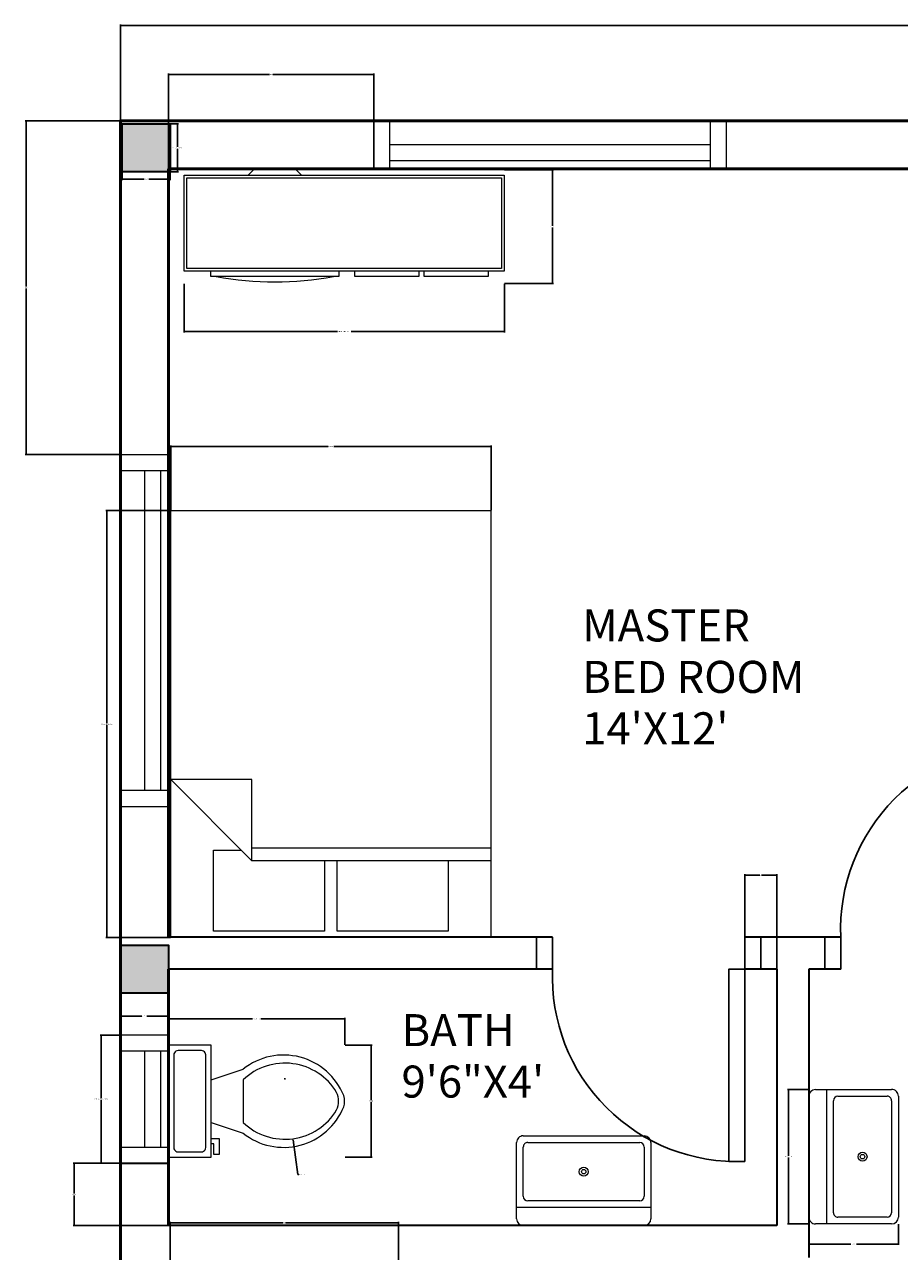
# Model space of a CAD drawing. Units: inches. Extents: x 2421 to 2780, y 382 to 769.
# Tile 3 of 4: x 2422 to 2585, y 539 to 769. Entities that reach past the tile are written whole.
import ezdxf

# ---------------------------------------------------------------- set-up
doc = ezdxf.new("R2010")
doc.units = ezdxf.units.IN
for name, color, linetype, lineweight in [('A-ANNO-DIMS', 2, 'Continuous', 18), ('A-AREA-IDEN', 7, 'Continuous', 25), ('A-COLS', 1, 'Continuous', 35), ('A-FLOR-FIXT', 3, 'Continuous', 18), ('DOOR', 1, 'Continuous', 25), ('FURNITURE', 3, 'Continuous', 18), ('INNER WALL', 2, 'Continuous', 35), ('OUTER WALL', 4, 'Continuous', 50), ('WINDOW', 5, 'Continuous', 18)]:
    doc.layers.add(name, color=color, linetype=linetype, lineweight=lineweight)
doc.styles.get("Standard").update_dxf_attribs({"font": 'arial.ttf'})
doc.dimstyles.get("Standard").update_dxf_attribs({"dimtxt": 0.18, "dimasz": 0.18, "dimexe": 0.18, "dimexo": 0.0625, "dimgap": 0.09, "dimtad": 0, "dimtih": 1, "dimtoh": 1, "dimdec": 4, "dimzin": 0, "dimdsep": 46, "dimtxsty": 'Standard', "dimcen": 0.09, "dimadec": 0, "dimazin": 0, "dimtfac": 1, "dimtdec": 4, "dimtofl": 0, "dimtmove": 0, "dimatfit": 3, "dimfxl": 1, "dimtolj": 1, "dimtzin": 0, "dimarcsym": 0})

# ---------------------------------------------------------------- blocks, each defined once
blk = doc.blocks.new('Bed - Queen')
for p, q in [((0, -80.00003), (0, 0)), ((0, 0), (59.99999, 0)), ((59.99999, 0), (59.99999, -80.00003)), ((7.99999, -1.2), (28.79998, -1.2)), ((7.99999, -14.4), (7.99999, -1.2)), ((28.79998, -1.2), (28.79998, -14.4)), ((31.19999, -1.2), (51.99999, -1.2)), ((31.19999, -14.4), (31.19999, -1.2)), ((51.99999, -1.2), (51.99999, -16.4)), ((0, -14.4), (44.8, -14.4)), ((59.99999, -29.6), (44.8, -14.4)), ((44.8, -14.4), (44.8, -29.6)), ((44.8, -16.8), (0, -16.8)), ((51.99999, -16.4), (46.79936, -16.4)), ((44.8, -29.6), (59.99999, -29.6)), ((59.99999, -80.00003), (0, -80.00003))]:
    blk.add_line(p, q)
blk = doc.blocks.new('Toilet - top')
for p, q in [((9.5, -6), (9.5, -2)), ((-10, -8.5), (-8, -8.5)), ((-10, -9.5), (-10, -8.5)), ((-8, -8.5), (-8, -8)), ((-7, -8), (-7, -9.5)), ((-4, -8), (-6, -14)), ((4, -8), (6, -14)), ((-7, -9.5), (-10, -9.5)), ((4, -14), (-4, -14))]:
    blk.add_line(p, q)
blk.add_lwpolyline([(10.5, -8), (10.5, 0), (-10.5, 0), (-10.5, -8)], close=True)
for points in [[(-9.5, -2), (-9.5, -6)], [(8.5, -1), (-8.5, -1)], [(-8.5, -7), (8.5, -7)]]:
    blk.add_lwpolyline(points)
for centre, radius, start, end in [((-8.62, -1.88), 0.884, 81.8699, 188.1301), ((8.62, -1.88), 0.884, 351.8699, 98.1301), ((-8.62, -6.12), 0.884, 171.8699, 278.1301), ((8.62, -6.12), 0.884, 261.8699, 8.1301), ((3.52, -21.58), 12.17, 141.4691, 247.9714), ((4.2, -21.82), 11.33, 136.3677, 238.9468), ((-3.52, -21.58), 12.17, 292.0284, 38.5307), ((-4.2, -21.82), 11.33, 301.053, 43.6321), ((0, -27.88), 4, 245.7318, 294.2682), ((0, -29), 4, 254.8605, 285.1395)]:
    blk.add_arc(centre, radius, start, end)
blk = doc.blocks.new('Entertainment Center')
for p, q in [((-4, 0), (-5, -1)), ((4, 0), (-4, 0)), ((5, -1), (4, 0)), ((-17, -19), (-17, -1)), ((-17, -1), (43, -1)), ((-16.5, -18.5), (-16.5, -1.5)), ((-16.5, -1.5), (42.5, -1.5)), ((42.5, -1.5), (42.5, -18.5)), ((43, -1), (43, -19)), ((43, -19), (-17, -19)), ((42.5, -18.5), (-16.5, -18.5)), ((-12, -20), (-12, -19)), ((12, -20), (-12, -20)), ((12, -19), (12, -20)), ((15, -20), (15, -19)), ((27, -20), (15, -20)), ((27, -19), (27, -20)), ((28, -20), (28, -19)), ((40, -20), (28, -20)), ((40, -19), (40, -20))]:
    blk.add_line(p, q)
blk.add_arc((0, 40), 61, 259.6111, 280.3889)
blk = doc.blocks.new('Sink-single - 30 in top')
blk.add_line((-15, -3.999996), (15, -3.999996))
for points in [[(-13.5, 0), (13.5, 0)], [(-15, -18.499996), (-15, -1.5)], [(15, -1.5), (15, -18.499996)], [(-13.5, -17.499996), (-13.5, -6.499996)], [(-12.5, -5.499996), (12.5, -5.499996)], [(13.5, -6.499996), (13.5, -17.499996)], [(12.5, -18.499996), (-12.5, -18.499996)], [(13.5, -19.999996), (-13.5, -19.999996)]]:
    blk.add_lwpolyline(points)
for radius in [1, 0.5]:
    blk.add_circle((0, -11.999996), radius)
for centre, radius, start, end in [((-13.5, -1.5), 1.5, 90, 180), ((13.5, -1.5), 1.5, 0, 90), ((-12.5, -6.499996), 1, 90, 180), ((12.5, -6.499996), 1, 0, 90), ((-13.5, -18.499996), 1.5, 180, 270), ((-12.5, -17.499996), 1, 180, 270), ((12.5, -17.499996), 1, 270, 0), ((13.5, -18.499996), 1.5, 270, 0)]:
    blk.add_arc(centre, radius, start, end)
blk = doc.blocks.new('DOOR-36IN-INT')
for p, q in [((0, 6), (0, 0)), ((3, 6), (3, 0)), ((39, 6), (39, 0)), ((42, 6), (42, 0))]:
    blk.add_line(p, q)
blk.add_lwpolyline([(3, 6), (6, 6), (6, 42), (3, 42)], close=True)
blk.add_arc((4.5, 7.5), 34.53, 357.5104, 92.4896)
blk = doc.blocks.new('WIN-60IN')
for p, q in [((0, 0), (0, 9)), ((3, 0), (3, 9)), ((63, 9), (63, 0)), ((66, 9), (66, 0)), ((63, 4.5), (3, 4.5)), ((63, 1.5), (3, 1.5))]:
    blk.add_line(p, q)
blk = doc.blocks.new('WIN-18IN')
for p, q in [((9, 24), (0, 24)), ((9, 21), (0, 21)), ((4.5, 21), (4.5, 3)), ((7.5, 21), (7.5, 3)), ((0, 3), (9, 3)), ((0, 0), (9, 0))]:
    blk.add_line(p, q)
blk = doc.blocks.new('COL-9X9IN')
h = blk.add_hatch(color=256)
h.dxf.hatch_style = 1
h.paths.add_polyline_path([(9, 9), (0, 9), (0, 0), (9, 0)])
blk.add_lwpolyline([(0, 9), (9, 9), (9, 0), (0, 0)], close=True)
blk = doc.blocks.new('*D18')
at = {"layer": 'A-ANNO-DIMS', "color": 0, "lineweight": -2, "transparency": 16777216}
for p, q in [((2448.87, 750.58), (2450.34, 750.58)), ((2450.16, 750.4), (2450.16, 746.27)), ((2450.16, 741.76), (2450.16, 745.9)), ((2448.87, 741.58), (2450.34, 741.58))]:
    blk.add_line(p, q, dxfattribs=at)
at = {"layer": 'A-ANNO-DIMS', "color": 0, "transparency": 16777216}
for points in [[(2450.13, 750.4), (2450.19, 750.4), (2450.16, 750.58)], [(2450.13, 741.76), (2450.19, 741.76), (2450.16, 741.58)]]:
    blk.add_solid(points, dxfattribs=at)
at = {"layer": 'Defpoints', "color": 0, "transparency": 16777216}
for p in [(2448.81, 750.58), (2450.16, 750.58), (2448.81, 741.58)]:
    blk.add_point(p, dxfattribs=at)
at = {"layer": 'A-ANNO-DIMS', "color": 0, "transparency": 16777216, "insert": (2450.16, 746.08), "char_height": 0.18, "attachment_point": 5}
blk.add_mtext('\\A1;COLUMN 9 TYP.', dxfattribs=at)
blk = doc.blocks.new('*D19')
at = {"layer": 'A-ANNO-DIMS', "color": 0, "lineweight": -2, "transparency": 16777216}
for p, q in [((2439.81, 741.52), (2439.81, 740.05)), ((2448.81, 741.52), (2448.81, 740.05)), ((2439.99, 740.23), (2443.85, 740.23)), ((2448.63, 740.23), (2444.77, 740.23))]:
    blk.add_line(p, q, dxfattribs=at)
at = {"layer": 'A-ANNO-DIMS', "color": 0, "transparency": 16777216}
for points in [[(2439.99, 740.26), (2439.99, 740.2), (2439.81, 740.23)], [(2448.63, 740.26), (2448.63, 740.2), (2448.81, 740.23)]]:
    blk.add_solid(points, dxfattribs=at)
at = {"layer": 'Defpoints', "color": 0, "transparency": 16777216}
for p in [(2439.81, 741.58), (2448.81, 741.58), (2448.81, 740.23)]:
    blk.add_point(p, dxfattribs=at)
at = {"layer": 'A-ANNO-DIMS', "color": 0, "transparency": 16777216, "insert": (2444.31, 740.23), "char_height": 0.18, "attachment_point": 5}
blk.add_mtext('\\A1;9 TYP.', dxfattribs=at)
blk = doc.blocks.new('*D22')
at = {"layer": 'A-ANNO-DIMS', "color": 0, "lineweight": -2, "transparency": 16777216}
for p, q in [((2439.4, 579.82), (2435.69, 579.82)), ((2435.87, 579.64), (2435.87, 568)), ((2435.87, 556), (2435.87, 567.63)), ((2439.4, 555.82), (2435.69, 555.82))]:
    blk.add_line(p, q, dxfattribs=at)
at = {"layer": 'A-ANNO-DIMS', "color": 0, "transparency": 16777216}
for points in [[(2435.84, 579.64), (2435.9, 579.64), (2435.87, 579.82)], [(2435.84, 556), (2435.9, 556), (2435.87, 555.82)]]:
    blk.add_solid(points, dxfattribs=at)
at = {"layer": 'Defpoints', "color": 0, "transparency": 16777216}
for p in [(2435.87, 579.82), (2439.47, 579.82), (2439.47, 555.82)]:
    blk.add_point(p, dxfattribs=at)
at = {"layer": 'A-ANNO-DIMS', "color": 0, "transparency": 16777216, "insert": (2435.87, 567.82), "char_height": 0.18, "attachment_point": 5}
blk.add_mtext('\\A1;BATH WINDOW 24 TYP.', dxfattribs=at)
blk = doc.blocks.new('*D23')
at = {"layer": 'A-ANNO-DIMS', "color": 0, "lineweight": -2, "transparency": 16777216}
for p, q in [((2439.47, 579.88), (2439.47, 583.6)), ((2439.65, 583.42), (2443.51, 583.42)), ((2448.29, 583.42), (2444.42, 583.42)), ((2448.47, 579.88), (2448.47, 583.6))]:
    blk.add_line(p, q, dxfattribs=at)
at = {"layer": 'A-ANNO-DIMS', "color": 0, "transparency": 16777216}
for points in [[(2439.65, 583.45), (2439.65, 583.39), (2439.47, 583.42)], [(2448.29, 583.45), (2448.29, 583.39), (2448.47, 583.42)]]:
    blk.add_solid(points, dxfattribs=at)
at = {"layer": 'Defpoints', "color": 0, "transparency": 16777216}
for p in [(2448.47, 583.42), (2439.47, 579.82), (2448.47, 579.82)]:
    blk.add_point(p, dxfattribs=at)
at = {"layer": 'A-ANNO-DIMS', "color": 0, "transparency": 16777216, "insert": (2443.97, 583.42), "char_height": 0.18, "attachment_point": 5}
blk.add_mtext('\\A1;9 TYP.', dxfattribs=at)
blk = doc.blocks.new('*D30')
at = {"layer": 'A-ANNO-DIMS', "color": 0, "lineweight": -2, "transparency": 16777216}
for p, q in [((2448.47, 578.02), (2448.47, 583.1)), ((2448.65, 582.92), (2464.22, 582.92)), ((2481.34, 582.92), (2465.77, 582.92)), ((2481.52, 578.02), (2481.52, 583.1))]:
    blk.add_line(p, q, dxfattribs=at)
at = {"layer": 'A-ANNO-DIMS', "color": 0, "transparency": 16777216}
for points in [[(2448.65, 582.95), (2448.65, 582.89), (2448.47, 582.92)], [(2481.34, 582.95), (2481.34, 582.89), (2481.52, 582.92)]]:
    blk.add_solid(points, dxfattribs=at)
at = {"layer": 'Defpoints', "color": 0, "transparency": 16777216}
for p in [(2448.47, 582.92), (2448.47, 577.96), (2481.52, 577.96)]:
    blk.add_point(p, dxfattribs=at)
at = {"layer": 'A-ANNO-DIMS', "color": 0, "transparency": 16777216, "insert": (2465, 582.92), "char_height": 0.18, "attachment_point": 5}
blk.add_mtext('\\A1;WC 33 TYP.', dxfattribs=at)
blk = doc.blocks.new('*D31')
at = {"layer": 'A-ANNO-DIMS', "color": 0, "lineweight": -2, "transparency": 16777216}
for p, q in [((2481.58, 577.96), (2486.66, 577.96)), ((2486.48, 577.78), (2486.48, 567.64)), ((2486.48, 557.14), (2486.48, 567.28)), ((2481.58, 556.96), (2486.66, 556.96))]:
    blk.add_line(p, q, dxfattribs=at)
at = {"layer": 'A-ANNO-DIMS', "color": 0, "transparency": 16777216}
for points in [[(2486.45, 577.78), (2486.51, 577.78), (2486.48, 577.96)], [(2486.45, 557.14), (2486.51, 557.14), (2486.48, 556.96)]]:
    blk.add_solid(points, dxfattribs=at)
at = {"layer": 'Defpoints', "color": 0, "transparency": 16777216}
for p in [(2481.52, 577.96), (2486.48, 577.96), (2481.52, 556.96)]:
    blk.add_point(p, dxfattribs=at)
at = {"layer": 'A-ANNO-DIMS', "color": 0, "transparency": 16777216, "insert": (2486.48, 567.46), "char_height": 0.18, "attachment_point": 5}
blk.add_mtext('\\A1;21 TYP.', dxfattribs=at)
blk = doc.blocks.new('*D32')
at = {"layer": 'A-ANNO-DIMS', "color": 0, "lineweight": -2, "transparency": 16777216}
for p, q in [((2448.86, 678.12), (2436.74, 678.12)), ((2436.92, 677.94), (2436.92, 638.31)), ((2436.92, 598.3), (2436.92, 637.93)), ((2448.86, 598.12), (2436.74, 598.12))]:
    blk.add_line(p, q, dxfattribs=at)
at = {"layer": 'A-ANNO-DIMS', "color": 0, "transparency": 16777216}
for points in [[(2436.89, 677.94), (2436.95, 677.94), (2436.92, 678.12)], [(2436.89, 598.3), (2436.95, 598.3), (2436.92, 598.12)]]:
    blk.add_solid(points, dxfattribs=at)
at = {"layer": 'Defpoints', "color": 0, "transparency": 16777216}
for p in [(2448.92, 678.12), (2436.92, 598.12), (2448.92, 598.12)]:
    blk.add_point(p, dxfattribs=at)
at = {"layer": 'A-ANNO-DIMS', "color": 0, "transparency": 16777216, "insert": (2436.92, 638.12), "char_height": 0.18, "attachment_point": 5}
blk.add_mtext('\\A1;QUEEN BED 80 TYP.', dxfattribs=at)
blk = doc.blocks.new('*D33')
at = {"layer": 'A-ANNO-DIMS', "color": 0, "lineweight": -2, "transparency": 16777216}
for p, q in [((2448.92, 678.18), (2448.92, 690.3)), ((2449.1, 690.12), (2478.39, 690.12)), ((2508.74, 690.12), (2479.45, 690.12)), ((2508.92, 678.18), (2508.92, 690.3))]:
    blk.add_line(p, q, dxfattribs=at)
at = {"layer": 'A-ANNO-DIMS', "color": 0, "transparency": 16777216}
for points in [[(2449.1, 690.15), (2449.1, 690.09), (2448.92, 690.12)], [(2508.74, 690.15), (2508.74, 690.09), (2508.92, 690.12)]]:
    blk.add_solid(points, dxfattribs=at)
at = {"layer": 'Defpoints', "color": 0, "transparency": 16777216}
for p in [(2448.92, 690.12), (2448.92, 678.12), (2508.92, 678.12)]:
    blk.add_point(p, dxfattribs=at)
at = {"layer": 'A-ANNO-DIMS', "color": 0, "transparency": 16777216, "insert": (2478.92, 690.12), "char_height": 0.18, "attachment_point": 5}
blk.add_mtext('\\A1;60 TYP.', dxfattribs=at)
blk = doc.blocks.new('*D34')
at = {"layer": 'A-ANNO-DIMS', "color": 0, "lineweight": -2, "transparency": 16777216}
for p, q in [((2451.42, 720.6), (2451.42, 711.48)), ((2511.42, 720.6), (2511.42, 711.48)), ((2451.6, 711.66), (2480.13, 711.66)), ((2511.24, 711.66), (2482.7, 711.66))]:
    blk.add_line(p, q, dxfattribs=at)
at = {"layer": 'A-ANNO-DIMS', "color": 0, "transparency": 16777216}
for points in [[(2451.6, 711.69), (2451.6, 711.63), (2451.42, 711.66)], [(2511.24, 711.69), (2511.24, 711.63), (2511.42, 711.66)]]:
    blk.add_solid(points, dxfattribs=at)
at = {"layer": 'Defpoints', "color": 0, "transparency": 16777216}
for p in [(2451.42, 720.66), (2511.42, 720.66), (2511.42, 711.66)]:
    blk.add_point(p, dxfattribs=at)
at = {"layer": 'A-ANNO-DIMS', "color": 0, "transparency": 16777216, "insert": (2481.42, 711.66), "char_height": 0.18, "attachment_point": 5}
blk.add_mtext('\\A1;MEDIA UNIT 60 TYP.', dxfattribs=at)
blk = doc.blocks.new('*D35')
at = {"layer": 'A-ANNO-DIMS', "color": 0, "lineweight": -2, "transparency": 16777216}
for p, q in [((2511.48, 742), (2520.6, 742)), ((2520.42, 741.82), (2520.42, 731.51)), ((2520.42, 720.84), (2520.42, 731.15)), ((2511.48, 720.66), (2520.6, 720.66))]:
    blk.add_line(p, q, dxfattribs=at)
at = {"layer": 'A-ANNO-DIMS', "color": 0, "transparency": 16777216}
for points in [[(2520.39, 741.82), (2520.45, 741.82), (2520.42, 742)], [(2520.39, 720.84), (2520.45, 720.84), (2520.42, 720.66)]]:
    blk.add_solid(points, dxfattribs=at)
at = {"layer": 'Defpoints', "color": 0, "transparency": 16777216}
for p in [(2511.42, 742), (2520.42, 742), (2511.42, 720.66)]:
    blk.add_point(p, dxfattribs=at)
at = {"layer": 'A-ANNO-DIMS', "color": 0, "transparency": 16777216, "insert": (2520.42, 731.33), "char_height": 0.18, "attachment_point": 5}
blk.add_mtext('\\A1;21 TYP.', dxfattribs=at)
blk = doc.blocks.new('*D36')
at = {"layer": 'A-ANNO-DIMS', "color": 0, "lineweight": -2, "transparency": 16777216}
for p, q in [((2568.4, 569.66), (2564.51, 569.66)), ((2564.69, 569.48), (2564.69, 557.25)), ((2564.69, 544.65), (2564.69, 556.88)), ((2568.4, 544.47), (2564.51, 544.47))]:
    blk.add_line(p, q, dxfattribs=at)
at = {"layer": 'A-ANNO-DIMS', "color": 0, "transparency": 16777216}
for points in [[(2564.66, 569.48), (2564.72, 569.48), (2564.69, 569.66)], [(2564.66, 544.65), (2564.72, 544.65), (2564.69, 544.47)]]:
    blk.add_solid(points, dxfattribs=at)
at = {"layer": 'Defpoints', "color": 0, "transparency": 16777216}
for p in [(2564.69, 569.66), (2568.47, 569.66), (2568.47, 544.47)]:
    blk.add_point(p, dxfattribs=at)
at = {"layer": 'A-ANNO-DIMS', "color": 0, "transparency": 16777216, "insert": (2564.69, 557.07), "char_height": 0.18, "attachment_point": 5}
blk.add_mtext('\\A1;BASIN 25 TYP.', dxfattribs=at)
blk = doc.blocks.new('*D37')
at = {"layer": 'A-ANNO-DIMS', "color": 0, "lineweight": -2, "transparency": 16777216}
for p, q in [((2568.47, 544.41), (2568.47, 540.52)), ((2585.25, 544.41), (2585.25, 540.52)), ((2568.65, 540.7), (2576.34, 540.7)), ((2585.07, 540.7), (2577.38, 540.7))]:
    blk.add_line(p, q, dxfattribs=at)
at = {"layer": 'A-ANNO-DIMS', "color": 0, "transparency": 16777216}
for points in [[(2568.65, 540.73), (2568.65, 540.67), (2568.47, 540.7)], [(2585.07, 540.73), (2585.07, 540.67), (2585.25, 540.7)]]:
    blk.add_solid(points, dxfattribs=at)
at = {"layer": 'Defpoints', "color": 0, "transparency": 16777216}
for p in [(2568.47, 544.47), (2585.25, 544.47), (2568.47, 540.7)]:
    blk.add_point(p, dxfattribs=at)
at = {"layer": 'A-ANNO-DIMS', "color": 0, "transparency": 16777216, "insert": (2576.86, 540.7), "char_height": 0.18, "attachment_point": 5}
blk.add_mtext('\\A1;17 TYP.', dxfattribs=at)
blk = doc.blocks.new('*D45')
at = {"layer": 'A-ANNO-DIMS', "color": 0, "lineweight": -2, "transparency": 16777216}
for p, q in [((2448.78, 537.5), (2448.78, 544.86)), ((2448.96, 544.68), (2469.97, 544.68)), ((2491.43, 544.68), (2470.42, 544.68)), ((2491.61, 537.5), (2491.61, 544.86))]:
    blk.add_line(p, q, dxfattribs=at)
at = {"layer": 'A-ANNO-DIMS', "color": 0, "transparency": 16777216}
for points in [[(2448.96, 544.71), (2448.96, 544.65), (2448.78, 544.68)], [(2491.43, 544.71), (2491.43, 544.65), (2491.61, 544.68)]]:
    blk.add_solid(points, dxfattribs=at)
at = {"layer": 'Defpoints', "color": 0, "transparency": 16777216}
for p in [(2448.78, 544.68), (2448.78, 537.44), (2491.61, 537.44)]:
    blk.add_point(p, dxfattribs=at)
at = {"layer": 'A-ANNO-DIMS', "color": 0, "transparency": 16777216, "insert": (2470.19, 544.68), "char_height": 0.18, "attachment_point": 5}
blk.add_mtext('\\A1;43', dxfattribs=at)
blk = doc.blocks.new('*D46')
at = {"layer": 'A-ANNO-DIMS', "color": 0, "lineweight": -2, "transparency": 16777216}
for p, q in [((2439.47, 751.24), (2439.47, 769.21)), ((2439.65, 769.03), (2595.18, 769.03)), ((2751.29, 769.03), (2595.75, 769.03)), ((2751.47, 751.24), (2751.47, 769.21))]:
    blk.add_line(p, q, dxfattribs=at)
at = {"layer": 'A-ANNO-DIMS', "color": 0, "transparency": 16777216}
for points in [[(2439.65, 769.06), (2439.65, 769), (2439.47, 769.03)], [(2751.29, 769.06), (2751.29, 769), (2751.47, 769.03)]]:
    blk.add_solid(points, dxfattribs=at)
at = {"layer": 'Defpoints', "color": 0, "transparency": 16777216}
for p in [(2751.47, 769.03), (2439.47, 751.18), (2751.47, 751.18)]:
    blk.add_point(p, dxfattribs=at)
at = {"layer": 'A-ANNO-DIMS', "color": 0, "transparency": 16777216, "insert": (2595.47, 769.03), "char_height": 0.18, "attachment_point": 5}
blk.add_mtext('\\A1;312', dxfattribs=at)
blk = doc.blocks.new('*D56')
at = {"layer": 'A-ANNO-DIMS', "color": 0, "lineweight": -2, "transparency": 16777216}
for p, q in [((2448.47, 742.24), (2448.47, 760.01)), ((2448.65, 759.83), (2467.39, 759.83)), ((2486.79, 759.83), (2468.04, 759.83)), ((2486.97, 742.24), (2486.97, 760.01))]:
    blk.add_line(p, q, dxfattribs=at)
at = {"layer": 'A-ANNO-DIMS', "color": 0, "transparency": 16777216}
for points in [[(2448.65, 759.86), (2448.65, 759.8), (2448.47, 759.83)], [(2486.79, 759.86), (2486.79, 759.8), (2486.97, 759.83)]]:
    blk.add_solid(points, dxfattribs=at)
at = {"layer": 'Defpoints', "color": 0, "transparency": 16777216}
for p in [(2486.97, 759.83), (2448.47, 742.18), (2486.97, 742.18)]:
    blk.add_point(p, dxfattribs=at)
at = {"layer": 'A-ANNO-DIMS', "color": 0, "transparency": 16777216, "insert": (2467.72, 759.83), "char_height": 0.18, "attachment_point": 5}
blk.add_mtext('\\A1;38.5', dxfattribs=at)
blk = doc.blocks.new('*D59')
at = {"layer": 'A-ANNO-DIMS', "color": 0, "lineweight": -2, "transparency": 16777216}
for p, q in [((2439.4, 751.18), (2421.64, 751.18)), ((2421.82, 751), (2421.82, 720.1)), ((2421.82, 688.83), (2421.82, 719.73)), ((2439.4, 688.65), (2421.64, 688.65))]:
    blk.add_line(p, q, dxfattribs=at)
at = {"layer": 'A-ANNO-DIMS', "color": 0, "transparency": 16777216}
for points in [[(2421.79, 751), (2421.85, 751), (2421.82, 751.18)], [(2421.79, 688.83), (2421.85, 688.83), (2421.82, 688.65)]]:
    blk.add_solid(points, dxfattribs=at)
at = {"layer": 'Defpoints', "color": 0, "transparency": 16777216}
for p in [(2421.82, 751.18), (2439.47, 751.18), (2439.47, 688.65)]:
    blk.add_point(p, dxfattribs=at)
at = {"layer": 'A-ANNO-DIMS', "color": 0, "transparency": 16777216, "insert": (2421.82, 719.91), "char_height": 0.18, "attachment_point": 5}
blk.add_mtext('\\A1;62.53', dxfattribs=at)
blk = doc.blocks.new('*D60')
at = {"layer": 'A-ANNO-DIMS', "color": 0, "lineweight": -2, "transparency": 16777216}
for p, q in [((2448.4, 555.82), (2430.64, 555.82)), ((2430.82, 555.64), (2430.82, 550.18)), ((2430.82, 544.36), (2430.82, 549.82)), ((2448.4, 544.18), (2430.64, 544.18))]:
    blk.add_line(p, q, dxfattribs=at)
at = {"layer": 'A-ANNO-DIMS', "color": 0, "transparency": 16777216}
for points in [[(2430.79, 555.64), (2430.85, 555.64), (2430.82, 555.82)], [(2430.79, 544.36), (2430.85, 544.36), (2430.82, 544.18)]]:
    blk.add_solid(points, dxfattribs=at)
at = {"layer": 'Defpoints', "color": 0, "transparency": 16777216}
for p in [(2430.82, 555.82), (2448.47, 555.82), (2448.47, 544.18)]:
    blk.add_point(p, dxfattribs=at)
at = {"layer": 'A-ANNO-DIMS', "color": 0, "transparency": 16777216, "insert": (2430.82, 550), "char_height": 0.18, "attachment_point": 5}
blk.add_mtext('\\A1;11.637', dxfattribs=at)
blk = doc.blocks.new('*D71')
at = {"layer": 'A-ANNO-DIMS', "color": 0, "lineweight": -2, "transparency": 16777216}
for p, q in [((2556.47, 592.24), (2556.47, 610.01)), ((2556.65, 609.83), (2559.32, 609.83)), ((2562.29, 609.83), (2559.62, 609.83)), ((2562.47, 592.24), (2562.47, 610.01))]:
    blk.add_line(p, q, dxfattribs=at)
at = {"layer": 'A-ANNO-DIMS', "color": 0, "transparency": 16777216}
for points in [[(2556.65, 609.86), (2556.65, 609.8), (2556.47, 609.83)], [(2562.29, 609.86), (2562.29, 609.8), (2562.47, 609.83)]]:
    blk.add_solid(points, dxfattribs=at)
at = {"layer": 'Defpoints', "color": 0, "transparency": 16777216}
for p in [(2562.47, 609.83), (2556.47, 592.18), (2562.47, 592.18)]:
    blk.add_point(p, dxfattribs=at)
at = {"layer": 'A-ANNO-DIMS', "color": 0, "transparency": 16777216, "insert": (2559.47, 609.83), "char_height": 0.18, "attachment_point": 5}
blk.add_mtext('\\A1;6', dxfattribs=at)
blk = doc.blocks.new('*D80')
at = {"layer": 'A-ANNO-DIMS', "color": 0, "lineweight": -2, "transparency": 16777216}
for p, q in [((2470.2, 571.66), (2470.38, 571.66)), ((2470.29, 571.57), (2470.29, 571.75)), ((2472.7, 553.7), (2471.82, 560.25)), ((2472.88, 553.7), (2472.7, 553.7))]:
    blk.add_line(p, q, dxfattribs=at)
at = {"layer": 'A-ANNO-DIMS', "color": 0, "transparency": 16777216}
blk.add_solid([(2471.85, 560.26), (2471.79, 560.25), (2471.8, 560.43)], dxfattribs=at)
at = {"layer": 'Defpoints', "color": 0, "transparency": 16777216}
for p in [(2470.29, 571.66), (2471.8, 560.43)]:
    blk.add_point(p, dxfattribs=at)
at = {"layer": 'A-ANNO-DIMS', "color": 0, "transparency": 16777216, "insert": (2473.56, 553.7), "char_height": 0.18, "attachment_point": 5}
blk.add_mtext('\\A1;4X R11.33', dxfattribs=at)

msp = doc.modelspace()

# ---------------------------------------------------------------- linework, layer by layer
at = {"layer": 'INNER WALL'}
for p, q in [((2520.466, 598.1806), (2448.466, 598.1806)), ((2574.466, 598.1806), (2556.466, 598.1806)), ((2520.466, 592.1806), (2448.466, 592.1806)), ((2562.466, 592.1806), (2556.466, 592.1806)), ((2562.466, 592.1806), (2562.466, 544.1806)), ((2568.466, 592.1806), (2568.466, 538.1806)), ((2574.466, 592.1806), (2568.466, 592.1806)), ((2562.466, 544.1806), (2448.466, 544.1806))]:
    msp.add_line(p, q, dxfattribs=at)
at = {"layer": 'OUTER WALL'}
for p, q in [((2448.466, 742.1806), (2448.466, 598.1806)), ((2616.466, 742.1806), (2448.466, 742.1806)), ((2448.466, 592.1806), (2448.466, 544.1806))]:
    msp.add_line(p, q, dxfattribs=at)
msp.add_lwpolyline([(2656.7381, 439.1806), (2751.466, 439.1806), (2751.466, 751.1806), (2439.466, 751.1806), (2439.466, 439.1806), (2620.7381, 439.1806)], dxfattribs=at)

# ---------------------------------------------------------------- block references
at = {"layer": 'A-COLS'}
for p in [(2439.8102, 741.5842), (2439.466, 587.6806)]:
    msp.add_blockref('COL-9X9IN', p, dxfattribs=at)
at = {"layer": 'A-FLOR-FIXT', "rotation": 90}
msp.add_blockref('Toilet - top', (2448.4721, 567.4605), dxfattribs=at)
at = {"layer": 'A-FLOR-FIXT', "xscale": 0.8393990052015698, "yscale": 0.8393990052015698, "zscale": 0.8393990052015698}
for p, rotation in [((2568.466, 557.0654), 89.99999999999999), ((2526.2986, 544.1806), 180)]:
    msp.add_blockref('Sink-single - 30 in top', p, dxfattribs=dict(at, rotation=rotation))
at = {"layer": 'DOOR', "extrusion": (0, 0, -1), "zscale": -1}
msp.add_blockref('DOOR-36IN-INT', (-2613.466, 592.1806), dxfattribs=at)
at = {"layer": 'DOOR', "rotation": 180}
msp.add_blockref('DOOR-36IN-INT', (2559.466, 598.1806), dxfattribs=at)
at = {"layer": 'FURNITURE'}
msp.add_blockref('Entertainment Center', (2468.4171, 741.9955), dxfattribs=at)
at = {"layer": 'FURNITURE', "rotation": 180}
msp.add_blockref('Bed - Queen', (2508.918, 598.1206), dxfattribs=at)
at = {"layer": 'WINDOW'}
for name, p in [('WIN-60IN', (2486.9694, 742.1806)), ('WIN-18IN', (2439.466, 555.818))]:
    msp.add_blockref(name, p, dxfattribs=at)
at = {"layer": 'WINDOW', "rotation": 89.99999999999989}
msp.add_blockref('WIN-60IN', (2448.466, 622.6485), dxfattribs=at)

# ---------------------------------------------------------------- texts
at = {"layer": 'A-AREA-IDEN'}
for s, p in [('MASTER', (2526.008, 653.6086)), ('BED ROOM', (2526.008, 643.9702)), ("14'X12'", (2526.008, 634.3317)), ('BATH', (2492.1447, 577.7748)), ('9\'6"X4\'', (2492.1447, 568.1363))]:
    msp.add_text(s, height=6, dxfattribs=at).set_placement(p)

# ---------------------------------------------------------------- dimensions: what is measured, and where the dimension line sits
at = {"layer": 'A-ANNO-DIMS'}
for base, p1, p2, override, picture, middle in [((2751.466, 769.0257), (2439.466, 751.1806), (2751.466, 751.1806), {"dimdec": 0, "dimlfac": 1, "dimrnd": 0, "dimzin": 0, "dimdsep": 46, "dimlunit": 2}, '*D46', (2595.466, 769.0257)), ((2486.9694, 759.8306), (2448.466, 742.1806), (2486.9694, 742.1806), {"dimdec": 1, "dimlfac": 1, "dimrnd": 0, "dimzin": 0, "dimdsep": 46, "dimlunit": 2}, '*D56', (2467.7177, 759.8306))]:
    dim = msp.add_linear_dim(base=base, p1=p1, p2=p2, dimstyle='Standard', override=override, dxfattribs=at)
    dim.commit()
    dim.dimension.update_dxf_attribs({"geometry": picture, "text_midpoint": middle})
for base, p1, p2, angle, override, picture, middle in [((2421.816, 751.1806), (2439.466, 688.6485), (2439.466, 751.1806), 90, {"dimdec": 2, "dimlfac": 1, "dimrnd": 0, "dimzin": 0, "dimdsep": 46, "dimlunit": 2}, '*D59', (2421.816, 719.9145)), ((2562.466, 609.8306), (2556.466, 592.1806), (2562.466, 592.1806), 0, {"dimdec": 0, "dimlfac": 1, "dimrnd": 0, "dimzin": 0, "dimdsep": 46, "dimlunit": 2}, '*D71', (2559.466, 609.8306)), ((2430.816, 555.818), (2448.466, 544.1806), (2448.466, 555.818), 90, {"dimdec": 3, "dimlfac": 1, "dimrnd": 0, "dimzin": 0, "dimdsep": 46, "dimlunit": 2}, '*D60', (2430.816, 549.9993)), ((2448.7819, 544.679), (2491.6068, 537.4352), (2448.7819, 537.4352), 180, {"dimdec": 0, "dimlfac": 1, "dimrnd": 0, "dimzin": 0, "dimdsep": 46, "dimlunit": 2}, '*D45', (2470.1943, 544.679))]:
    dim = msp.add_linear_dim(base=base, p1=p1, p2=p2, angle=angle, dimstyle='Standard', override=override, dxfattribs=at)
    dim.commit()
    dim.dimension.update_dxf_attribs({"geometry": picture, "text_midpoint": middle})
for base, p1, p2, angle, text, picture, middle in [((2450.1602, 750.5842), (2448.8102, 741.5842), (2448.8102, 750.5842), 90, 'COLUMN <> TYP.', '*D18', (2450.1602, 746.0842)), ((2520.4171, 741.9955), (2511.4171, 720.6622), (2511.4171, 741.9955), 90, '<> TYP.', '*D35', (2520.4171, 731.3289)), ((2448.918, 690.1206), (2508.918, 678.1206), (2448.918, 678.1206), 180, '<> TYP.', '*D33', (2478.918, 690.1206)), ((2436.918, 598.1206), (2448.918, 678.1206), (2448.918, 598.1206), 270, 'QUEEN BED <> TYP.', '*D32', (2436.918, 638.1206)), ((2448.4721, 582.9174), (2481.5184, 577.9605), (2448.4721, 577.9605), 180, 'WC <> TYP.', '*D30', (2464.9952, 582.9174)), ((2435.866, 579.818), (2439.466, 555.818), (2439.466, 579.818), 90, 'BATH WINDOW <> TYP.', '*D22', (2435.866, 567.818)), ((2486.4753, 577.9605), (2481.5184, 556.9605), (2481.5184, 577.9605), 90, '<> TYP.', '*D31', (2486.4753, 567.4605)), ((2564.6887, 569.6564), (2568.466, 544.4744), (2568.466, 569.6564), 90, 'BASIN <> TYP.', '*D36', (2564.6887, 557.0654)), ((2568.466, 540.6971), (2585.254, 544.4744), (2568.466, 544.4744), 180, '<> TYP.', '*D37', (2576.86, 540.6971))]:
    dim = msp.add_linear_dim(base=base, p1=p1, p2=p2, angle=angle, text=text, dimstyle='Standard', override={"dimdec": 0, "dimlfac": 1, "dimrnd": 0, "dimzin": 0, "dimdsep": 46, "dimlunit": 2}, dxfattribs=at)
    dim.commit()
    dim.dimension.update_dxf_attribs({"geometry": picture, "text_midpoint": middle})
for base, p1, p2, text, picture, middle in [((2448.8102, 740.2342), (2439.8102, 741.5842), (2448.8102, 741.5842), '<> TYP.', '*D19', (2444.3102, 740.2342)), ((2511.4171, 711.6622), (2451.4171, 720.6622), (2511.4171, 720.6622), 'MEDIA UNIT <> TYP.', '*D34', (2481.4171, 711.6622)), ((2448.466, 583.418), (2439.466, 579.818), (2448.466, 579.818), '<> TYP.', '*D23', (2443.966, 583.418))]:
    dim = msp.add_linear_dim(base=base, p1=p1, p2=p2, text=text, dimstyle='Standard', override={"dimdec": 0, "dimlfac": 1, "dimrnd": 0, "dimzin": 0, "dimdsep": 46, "dimlunit": 2}, dxfattribs=at)
    dim.commit()
    dim.dimension.update_dxf_attribs({"geometry": picture, "text_midpoint": middle})
dim = msp.add_radius_dim(center=(2470.2895, 571.6604), mpoint=(2471.799, 560.4323), text='4X <>', dimstyle='Standard', override={"dimdec": 2, "dimlfac": 1, "dimrnd": 0, "dimzin": 0, "dimdsep": 46, "dimlunit": 2}, dxfattribs=at)
dim.commit()
dim.dimension.update_dxf_attribs({"geometry": '*D80', "text_midpoint": (2473.5615, 553.6954), "dimtype": 164})

doc.saveas('drawing.dxf')
